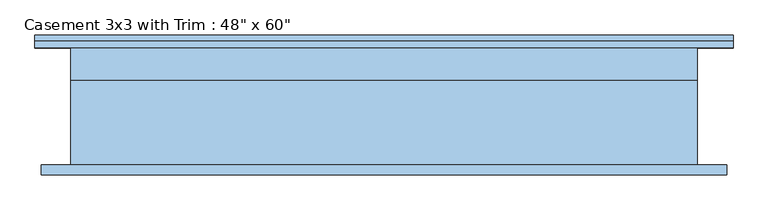
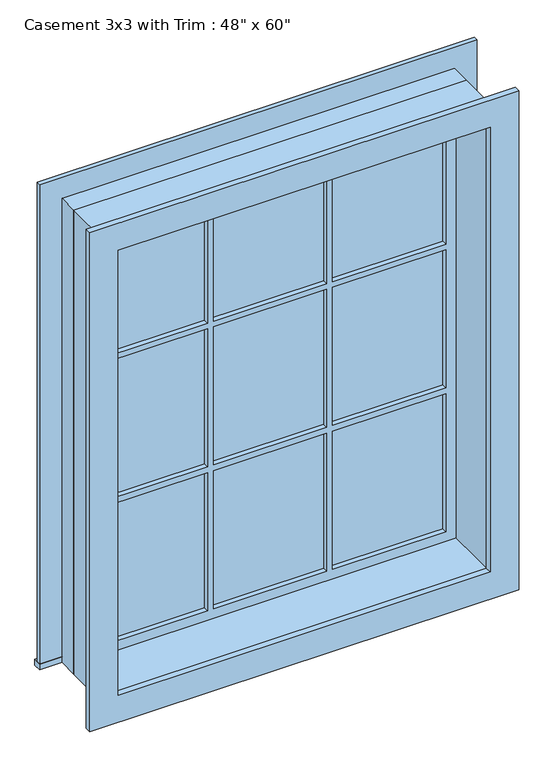
"""IFC4 building model written with IfcOpenShell, lengths in millimetres: window geometry."""

from ifc_helpers import new_model, si_unit, frame, origin, place, context, project, spatial, polyline, outline, extrude, source, transform, mapped, element, save


def window_544f1267(model_context):
    return source(origin(), model_context, "Body", "SweptSolid", [
        extrude(outline(polyline([(-679.45, 139.7), (679.45, 139.7), (679.45, 114.3), (-679.45, 114.3), (-679.45, 139.7)])), frame((0.0, 0.0, 304.8), z_axis=(0.0, 0.0, 1.0), x_axis=(1.0, 0.0, 0.0)), (0.0, 0.0, 1.0), 19.05),
        extrude(outline(polyline([(1809.75, -590.55), (1809.75, 590.55), (323.85, 590.55), (323.85, 679.45), (1898.65, 679.45), (1898.65, -679.45), (323.85, -679.45), (323.85, -590.55), (1809.75, -590.55)])), frame((0.0, 114.3, 0.0), z_axis=(0.0, 1.0, 0.0), x_axis=(0.0, 0.0, 1.0)), (0.0, 0.0, 1.0), 12.7),
        extrude(outline(polyline([(194.7333333, 79.375), (546.1, 79.375), (546.1, 66.675), (194.7333333, 66.675), (194.7333333, 79.375)])), frame((0.0, 0.0, 1312.3333333), z_axis=(0.0, 0.0, 1.0), x_axis=(1.0, 0.0, 0.0)), (0.0, 0.0, 1.0), 452.9666667),
        extrude(outline(polyline([(-175.6833333, 79.375), (175.6833333, 79.375), (175.6833333, 66.675), (-175.6833333, 66.675), (-175.6833333, 79.375)])), frame((0.0, 0.0, 1312.3333333), z_axis=(0.0, 0.0, 1.0), x_axis=(1.0, 0.0, 0.0)), (0.0, 0.0, 1.0), 452.9666667),
        extrude(outline(polyline([(-546.1, 79.375), (-194.7333333, 79.375), (-194.7333333, 66.675), (-546.1, 66.675), (-546.1, 79.375)])), frame((0.0, 0.0, 1312.3333333), z_axis=(0.0, 0.0, 1.0), x_axis=(1.0, 0.0, 0.0)), (0.0, 0.0, 1.0), 452.9666667),
        extrude(outline(polyline([(-546.1, 79.375), (-194.7333333, 79.375), (-194.7333333, 66.675), (-546.1, 66.675), (-546.1, 79.375)])), frame((0.0, 0.0, 840.3166667), z_axis=(0.0, 0.0, 1.0), x_axis=(1.0, 0.0, 0.0)), (0.0, 0.0, 1.0), 452.9666667),
        extrude(outline(polyline([(-175.6833333, 79.375), (175.6833333, 79.375), (175.6833333, 66.675), (-175.6833333, 66.675), (-175.6833333, 79.375)])), frame((0.0, 0.0, 840.3166667), z_axis=(0.0, 0.0, 1.0), x_axis=(1.0, 0.0, 0.0)), (0.0, 0.0, 1.0), 452.9666667),
        extrude(outline(polyline([(194.7333333, 79.375), (546.1, 79.375), (546.1, 66.675), (194.7333333, 66.675), (194.7333333, 79.375)])), frame((0.0, 0.0, 840.3166667), z_axis=(0.0, 0.0, 1.0), x_axis=(1.0, 0.0, 0.0)), (0.0, 0.0, 1.0), 452.9666667),
        extrude(outline(polyline([(194.7333333, 79.375), (546.1, 79.375), (546.1, 66.675), (194.7333333, 66.675), (194.7333333, 79.375)])), frame((0.0, 0.0, 368.3), z_axis=(0.0, 0.0, 1.0), x_axis=(1.0, 0.0, 0.0)), (0.0, 0.0, 1.0), 452.9666667),
        extrude(outline(polyline([(-175.6833333, 79.375), (175.6833333, 79.375), (175.6833333, 66.675), (-175.6833333, 66.675), (-175.6833333, 79.375)])), frame((0.0, 0.0, 368.3), z_axis=(0.0, 0.0, 1.0), x_axis=(1.0, 0.0, 0.0)), (0.0, 0.0, 1.0), 452.9666667),
        extrude(outline(polyline([(-546.1, 79.375), (-194.7333333, 79.375), (-194.7333333, 66.675), (-546.1, 66.675), (-546.1, 79.375)])), frame((0.0, 0.0, 368.3), z_axis=(0.0, 0.0, 1.0), x_axis=(1.0, 0.0, 0.0)), (0.0, 0.0, 1.0), 452.9666667),
        extrude(outline(polyline([(1885.95, 666.75), (1885.95, -666.75), (247.65, -666.75), (247.65, 666.75), (1885.95, 666.75)]), holes=[polyline([(1797.05, 577.85), (336.55, 577.85), (336.55, -577.85), (1797.05, -577.85), (1797.05, 577.85)])]), frame((0.0, -133.35, 0.0), z_axis=(0.0, 1.0, 0.0), x_axis=(0.0, 0.0, 1.0)), (0.0, 0.0, 1.0), 19.05),
        extrude(outline(polyline([(1809.75, -590.55), (323.85, -590.55), (323.85, 590.55), (1809.75, 590.55), (1809.75, -590.55)]), holes=[polyline([(1765.3, -194.7333333), (1312.3333333, -194.7333333), (1312.3333333, -546.1), (1765.3, -546.1), (1765.3, -194.7333333)]), polyline([(1293.2833333, -194.7333333), (840.3166667, -194.7333333), (840.3166667, -546.1), (1293.2833333, -546.1), (1293.2833333, -194.7333333)]), polyline([(821.2666667, -194.7333333), (368.3, -194.7333333), (368.3, -546.1), (821.2666667, -546.1), (821.2666667, -194.7333333)]), polyline([(1765.3, 175.6833333), (1312.3333333, 175.6833333), (1312.3333333, -175.6833333), (1765.3, -175.6833333), (1765.3, 175.6833333)]), polyline([(1293.2833333, 175.6833333), (840.3166667, 175.6833333), (840.3166667, -175.6833333), (1293.2833333, -175.6833333), (1293.2833333, 175.6833333)]), polyline([(821.2666667, 175.6833333), (368.3, 175.6833333), (368.3, -175.6833333), (821.2666667, -175.6833333), (821.2666667, 175.6833333)]), polyline([(1765.3, 546.1), (1312.3333333, 546.1), (1312.3333333, 194.7333333), (1765.3, 194.7333333), (1765.3, 546.1)]), polyline([(1293.2833333, 546.1), (840.3166667, 546.1), (840.3166667, 194.7333333), (1293.2833333, 194.7333333), (1293.2833333, 546.1)]), polyline([(821.2666667, 546.1), (368.3, 546.1), (368.3, 194.7333333), (821.2666667, 194.7333333), (821.2666667, 546.1)])]), frame((0.0, 50.8, 0.0), z_axis=(0.0, 1.0, 0.0), x_axis=(0.0, 0.0, 1.0)), (0.0, 0.0, 1.0), 44.45),
        extrude(outline(polyline([(1828.8, -609.6), (304.8, -609.6), (304.8, 609.6), (1828.8, 609.6), (1828.8, -609.6)]), holes=[polyline([(1797.05, -577.85), (1797.05, 577.85), (336.55, 577.85), (336.55, -577.85), (1797.05, -577.85)])]), frame((0.0, -114.3, 0.0), z_axis=(0.0, 1.0, 0.0), x_axis=(0.0, 0.0, 1.0)), (0.0, 0.0, 1.0), 165.1),
        extrude(outline(polyline([(1828.8, 609.6), (1828.8, -609.6), (304.8, -609.6), (304.8, 609.6), (1828.8, 609.6)]), holes=[polyline([(1809.75, 590.55), (323.85, 590.55), (323.85, -590.55), (1809.75, -590.55), (1809.75, 590.55)])]), frame((0.0, 50.8, 0.0), z_axis=(0.0, 1.0, 0.0), x_axis=(0.0, 0.0, 1.0)), (0.0, 0.0, 1.0), 63.5),
    ])


if __name__ == "__main__":
    model = new_model("IFC4")
    model_context = context("Model", 3, world=origin())
    ifc_project = project(units=[si_unit("LENGTHUNIT", "METRE", prefix="MILLI")], contexts=[model_context])
    site = spatial("IfcSite", under=ifc_project)
    building = spatial("IfcBuilding", under=site)
    placement = place(None, origin())
    window_shape = window_544f1267(model_context)
    element("IfcWindow", 1, ObjectType="Casement 3x3 with Trim : 48\" x 60\"", at=placement, inside=building, context=model_context, shape_type="MappedRepresentation", body=[
        mapped(window_shape, transform((0.0, 0.0, 0.0), x_axis=(1.0, 0.0, 0.0), y_axis=(0.0, 1.0, 0.0), z_axis=(0.0, 0.0, 1.0))),
    ])
    save(model, "model.ifc")

# Revit data of these elements
# Type "Casement 3x3 with Trim : 48\" x 60\""
#   Type Mark = "12"
#   Construction Type Id = "GSP4R"
#   Assembly Code = "B2020100"
#   Analytic Construction = "1/8 in Pilkington single glazing"
#   Visual Light Transmittance = 0.9
#   Solar Heat Gain Coefficient = 0.78
#   Heat Transfer Coefficient (U) = 0.6496 BTU/(h·ft²·°F)
#   Height = 5' - 0"
#   Default Sill Height = 1' - 0"
#   Trim Projection - Ext. = 0' - 0 1/2"
#   Trim Projection - Int. = 0' - 0 3/4"
#   Trim Width - Exterior = 0' - 3 1/2"
#   Trim Width - Interior = 0' - 3 1/2"
#   Width = 4' - 0"
#   Window Inset = 0' - 0 3/4"
#   Define Thermal Properties by = 1
#   Glass Pane Material = Glass
#   Sash Material = Sash
#   Trim Exterior Material = Trim
#   Trim Interior Material = Trim
#   Wall Closure = (empty or 0)
# Element 1 (IfcWindow, "Casement 3x3 with Trim : 48\" x 60\"")
#   Materials on its faces: "Sash", "Glass", "Trim"
# Materials
#   "Glass": class "Glass", colour RGB 0 128 192, transparency 0.75, Description = "Soda Lime Glass", Cost = 0
#   "Sash": class "Wood", colour RGB 224 178 126, transparency 0
#   "Trim": class "Wood", colour RGB 224 178 126, transparency 0
